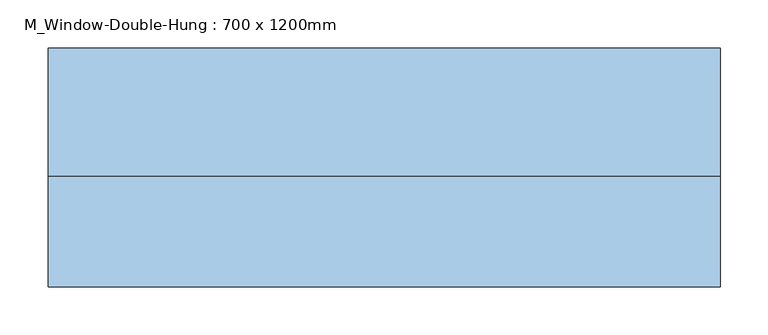
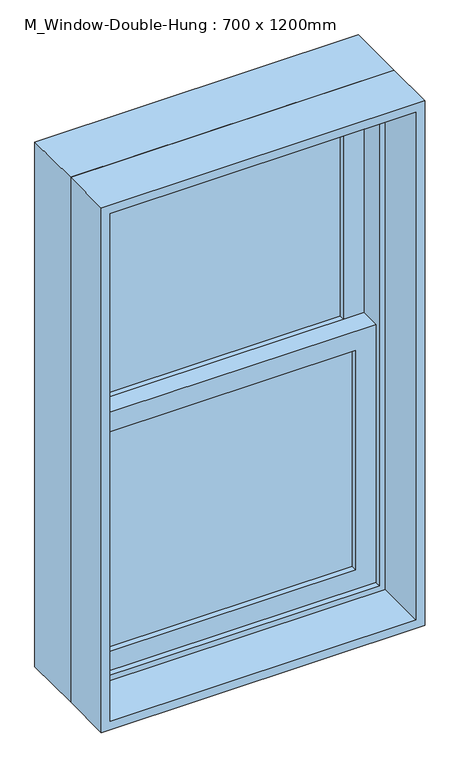
"""IFC4 building model written with IfcOpenShell, lengths in millimetres: window geometry, M_Window-Double-Hung : 700 x 1200mm."""

from ifc_helpers import new_model, si_unit, frame, origin, place, context, project, spatial, polyline, outline, extrude, source, transform, mapped, element, save


def m_window_double_hung_700_x_1200mm_3a464380(model_context):
    return source(origin(), model_context, "Body", "SweptSolid", [
        extrude(outline(polyline([(273.8, 45.15), (273.8, 38.8), (-273.8, 38.8), (-273.8, 45.15), (273.8, 45.15)])), frame((0.0, 0.0, 990.6), z_axis=(0.0, 0.0, 1.0), x_axis=(1.0, 0.0, 0.0)), (0.0, 0.0, 1.0), 501.575),
        extrude(outline(polyline([(-273.8, 32.45), (273.8, 32.45), (273.8, 26.1), (-273.8, 26.1), (-273.8, 32.45)])), frame((0.0, 0.0, 990.6), z_axis=(0.0, 0.0, 1.0), x_axis=(1.0, 0.0, 0.0)), (0.0, 0.0, 1.0), 501.575),
        extrude(outline(polyline([(273.8, 89.6), (273.8, 83.25), (-273.8, 83.25), (-273.8, 89.6), (273.8, 89.6)])), frame((0.0, 0.0, 1536.625), z_axis=(0.0, 0.0, 1.0), x_axis=(1.0, 0.0, 0.0)), (0.0, 0.0, 1.0), 501.575),
        extrude(outline(polyline([(-273.8, 76.9), (273.8, 76.9), (273.8, 70.55), (-273.8, 70.55), (-273.8, 76.9)])), frame((0.0, 0.0, 1536.625), z_axis=(0.0, 0.0, 1.0), x_axis=(1.0, 0.0, 0.0)), (0.0, 0.0, 1.0), 501.575),
        extrude(outline(polyline([(1536.625, -318.25), (946.15, -318.25), (946.15, 318.25), (1536.625, 318.25), (1536.625, -318.25)]), holes=[polyline([(1492.175, 273.8), (990.6, 273.8), (990.6, -273.8), (1492.175, -273.8), (1492.175, 273.8)])]), frame((0.0, 13.4, 0.0), z_axis=(0.0, 1.0, 0.0), x_axis=(0.0, 0.0, 1.0)), (0.0, 0.0, 1.0), 44.45),
        extrude(outline(polyline([(2082.65, -318.25), (1492.175, -318.25), (1492.175, 318.25), (2082.65, 318.25), (2082.65, -318.25)]), holes=[polyline([(2038.2, 273.8), (1536.625, 273.8), (1536.625, -273.8), (2038.2, -273.8), (2038.2, 273.8)])]), frame((0.0, 57.85, 0.0), z_axis=(0.0, 1.0, 0.0), x_axis=(0.0, 0.0, 1.0)), (0.0, 0.0, 1.0), 44.45),
        extrude(outline(polyline([(2114.4, -350.0), (914.4, -350.0), (914.4, 350.0), (2114.4, 350.0), (2114.4, -350.0)]), holes=[polyline([(2082.65, 318.25), (946.15, 318.25), (946.15, -318.25), (2082.65, -318.25), (2082.65, 318.25)])]), frame((0.0, 0.7, 0.0), z_axis=(0.0, 1.0, 0.0), x_axis=(0.0, 0.0, 1.0)), (0.0, 0.0, 1.0), 133.35),
        extrude(outline(polyline([(2114.4, 350.0), (2114.4, -350.0), (914.4, -350.0), (914.4, 350.0), (2114.4, 350.0)]), holes=[polyline([(2095.35, 330.95), (933.45, 330.95), (933.45, -330.95), (2095.35, -330.95), (2095.35, 330.95)])]), frame((0.0, -115.0, 0.0), z_axis=(0.0, 1.0, 0.0), x_axis=(0.0, 0.0, 1.0)), (0.0, 0.0, 1.0), 115.7),
    ])


if __name__ == "__main__":
    model = new_model("IFC4")
    model_context = context("Model", 3, world=origin())
    ifc_project = project(units=[si_unit("LENGTHUNIT", "METRE", prefix="MILLI")], contexts=[model_context])
    site = spatial("IfcSite", under=ifc_project)
    building = spatial("IfcBuilding", under=site)
    placement = place(None, origin())
    m_window_double_hung_700_x_1200mm_shape = m_window_double_hung_700_x_1200mm_3a464380(model_context)
    element("IfcWindow", 1, ObjectType="M_Window-Double-Hung : 700 x 1200mm", at=placement, inside=building, context=model_context, shape_type="MappedRepresentation", body=[
        mapped(m_window_double_hung_700_x_1200mm_shape, transform((0.0, 0.0, 0.0), x_axis=(1.0, 0.0, 0.0), y_axis=(0.0, 1.0, 0.0), z_axis=(0.0, 0.0, 1.0))),
    ])
    save(model, "model.ifc")

# Revit data of these elements
# Type "M_Window-Double-Hung : 700 x 1200mm"
#   Type Mark = "W3"
#   Fire Rating = "0.5h"
#   Construction Type Id = "DG-DR"
#   Assembly Code = "B2020100"
#   Analytic Construction = "Double glazing - domestic"
#   Wall Thickness [instance default] = 0.15 m
#   Window Inset [instance default] = 0 m
#   Visual Light Transmittance = 0.81
#   Thermal Resistance (R) = 0.319569 (m²·K)/W
#   Solar Heat Gain Coefficient = 0.76
#   Muntin Width = 0.5476 m
#   Muntin Height = 0.501575 m
#   Interior Wall Closure [instance default] = 0.0357 m
#   Rough Width = 0.715 m
#   Rough Height = 1.215 m
#   Frame Extension [instance default] = 0.03175 m
#   Exterior Wall Closure [instance default] = 0.0127 m
#   Extension Jamb [instance default] = 0.0357 m
#   Heat Transfer Coefficient (U) = 3.12929 W/(m²·K)
#   Height = 1.2 m
#   Width = 0.7 m
#   Define Thermal Properties by = 1
#   Top Muntin Visibility = yes
#   Indicator Visibility [instance default] = yes
#   Extension Jamb Visibility [instance default] = yes
#   Interior Trim Visibility [instance default] = yes
#   Exterior Trim Visibility [instance default] = yes
#   Define Thermal Properties by = 1
#   Bottom Muntin Visibility = yes
#   Muntin Pattern = M_Muntin Pattern_2x2 : M_Muntin Pattern_2x2
#   Interior Trim Material = Wood - Stained
#   Interior Trim = M_Trim-Window-Interior-Flat : Picture Frame
#   Exterior Trim Material = Clad - White
#   Exterior Trim = M_Trim-Window-Exterior-Flat : with Sill
#   Glass Panel Material = Glass
#   Exterior Frame Material = Clad - White
#   Interior Frame Material = Wood - Stained
#   Wall Closure = (empty or 0)
# Element 1 (IfcWindow, "M_Window-Double-Hung : 700 x 1200mm")
#   Wall Thickness = 0.23 m
#   Extension Jamb = 0.1157 m
#   Materials on its faces: "Wood - Stained", "Glass", "Clad - White"
# Materials
#   "Wood - Stained": class "Wood", colour RGB 224 178 126, transparency 0, Cost = 0
#   "Clad - White": class "Wood", colour RGB 242 242 238, transparency 0, Cost = 0
#   "Glass": class "Glass", colour RGB 0 128 192, transparency 0.9, Description = "Soda Lime Glass", Cost = 0
